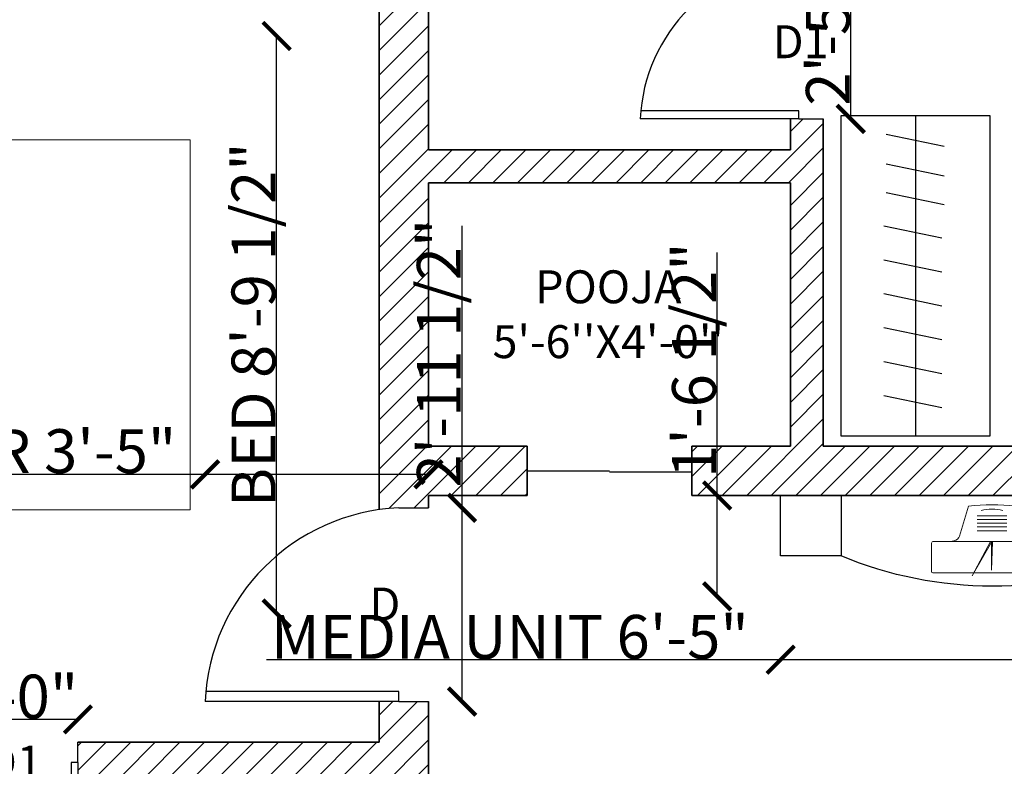
# Model space of a CAD drawing. Units: inches. Extents: x 2094 to 2639, y 1426 to 1997.
# Tile 6 of 8: x 2243 to 2423, y 1730 to 1866. Entities that reach past the tile are written whole.
import ezdxf

# ---------------------------------------------------------------- set-up
doc = ezdxf.new("R2010")
doc.units = ezdxf.units.IN
for name, color, linetype, lineweight in [('A-ANNO-DIMS', 2, 'Continuous', 18), ('A-ANNO-TEXT', 7, 'Continuous', 18), ('A-AREA-IDEN', 7, 'Continuous', 25), ('A-FLOR-CASE', 8, 'Continuous', 25), ('A-FURN', 8, 'Continuous', 18), ('A-WALL-PATT', 8, 'Continuous', 13), ('Doors', 34, 'Continuous', 25), ('Walls', 7, 'Continuous', 35)]:
    doc.layers.add(name, color=color, linetype=linetype, lineweight=lineweight)
doc.layers.add('THIET-BI', color=21, linetype='Continuous')
doc.styles.get("Standard").update_dxf_attribs({"font": 'arial.ttf'})
doc.dimstyles.get("Standard").update_dxf_attribs({"dimtxt": 8, "dimasz": 5, "dimexe": 0.18, "dimexo": 0.0625, "dimgap": 0.09, "dimtad": 1, "dimdec": 1, "dimzin": 0, "dimdsep": 46, "dimlunit": 4, "dimtxsty": 'Standard', "dimblk": 'ARCHTICK', "dimcen": 0.09, "dimse1": 1, "dimse2": 1, "dimadec": 0, "dimazin": 0, "dimtfac": 1, "dimtdec": 1, "dimtofl": 0, "dimtmove": 0, "dimatfit": 3, "dimfxl": 1, "dimtolj": 1, "dimtzin": 0, "dimarcsym": 0})

# ---------------------------------------------------------------- blocks, each defined once
blk = doc.blocks.new('AP0B05')
for p, q in [((35, 100), (35, 880)), ((75, 100), (75, 878.9)), ((35, 100), (35, -20)), ((815, 100), (815, -20))]:
    blk.add_line(p, q)
blk.add_lwpolyline([(35, 100), (75, 100)])
blk.add_arc((-2.4, 62.6), 818.3, 2.6212, 87.3788)
blk = doc.blocks.new('*X3')
at = {"color": 0}
for p, q in [((20.25, 14.8125), (20.2772, 14.8125)), ((20.1875, 14.75), (20.1875, 14.7669)), ((20.199, 14.7812), (20.2772, 14.7812)), ((20.1562, 14.625), (20.1562, 14.7281)), ((20.1739, 14.75), (20.2772, 14.75)), ((20.25, 14.3194), (20.25, 14.75)), ((20.1236, 14.6875), (20.25, 14.6875)), ((20.125, 14.5), (20.125, 14.6893)), ((20.1487, 14.7188), (20.2772, 14.7188)), ((20.0938, 14.375), (20.0938, 14.6504)), ((20.0984, 14.6562), (20.125, 14.6562)), ((20.0625, 14.2573), (20.0625, 14.6116)), ((20.2188, 14.3091), (20.2188, 14.625)), ((20.25, 14.625), (20.2772, 14.625)), ((20.0312, 14.2469), (20.0312, 14.5727)), ((20.125, 14.5938), (20.2772, 14.5938)), ((19.9979, 14.5312), (20.2772, 14.5312)), ((20.023, 14.5625), (20.2772, 14.5625)), ((19.9727, 14.5), (20.25, 14.5)), ((20, 14.2366), (20, 14.5)), ((20.1875, 14.2987), (20.1875, 14.5)), ((19.9476, 14.4688), (20.125, 14.4688)), ((19.9062, 14.375), (19.9062, 14.4174)), ((19.9225, 14.4375), (20, 14.4375)), ((20.125, 14.4062), (20.2772, 14.4062)), ((20.25, 14.4375), (20.2772, 14.4375)), ((19.875, 14.25), (19.875, 14.3785)), ((19.9688, 14.2262), (19.9688, 14.375)), ((20, 14.375), (20.2772, 14.375)), ((20.1562, 14.2884), (20.1562, 14.375)), ((19.8438, 14.1848), (19.8438, 14.3397)), ((19.875, 14.3438), (20.2772, 14.3438)), ((19.8125, 14.1744), (19.8125, 14.3008)), ((19.8219, 14.3125), (20.2291, 14.3125)), ((19.7716, 14.25), (20, 14.25)), ((19.7812, 14.1641), (19.7812, 14.262)), ((19.7967, 14.2812), (20.125, 14.2812)), ((19.9375, 14.2159), (19.9375, 14.25)), ((19.7465, 14.2188), (19.875, 14.2188)), ((19.75, 14.1537), (19.75, 14.2231)), ((19.7213, 14.1875), (19.75, 14.1875)), ((19.7018, 14.0938), (19.7786, 14.0938)), ((19.7188, 14.0726), (19.7188, 14.1136)), ((19.75, 14.0338), (19.75, 14.1032)), ((19.7812, 13.9949), (19.7812, 14.0929)), ((19.7269, 14.0625), (19.8728, 14.0625)), ((19.8125, 14), (19.8125, 14.0825)), ((19.9062, 13.8396), (19.9062, 14.0514)), ((19.752, 14.0312), (19.875, 14.0312)), ((19.9375, 13.8007), (19.9375, 14.0411)), ((19.9688, 13.875), (19.9688, 14.0307)), ((20, 14), (20, 14.0204)), ((19.875, 13.8784), (19.875, 14)), ((19.875, 13.9688), (20.1557, 13.9688)), ((20, 14), (20.0614, 14)), ((20.0625, 13.6454), (20.0625, 13.9996)), ((20.0938, 13.625), (20.0938, 13.9893)), ((20.125, 13.75), (20.125, 13.9789)), ((20.1562, 13.875), (20.1562, 13.9686)), ((19.8275, 13.9375), (20.25, 13.9375)), ((20.25, 13.5), (20.25, 13.9375)), ((19.8526, 13.9062), (20.125, 13.9062)), ((19.8777, 13.875), (20, 13.875)), ((20.0312, 13.6842), (20.0312, 13.875)), ((20.2188, 13.4511), (20.2188, 13.875)), ((20.25, 13.875), (20.2772, 13.875)), ((20, 13.8125), (20.2772, 13.8125)), ((20.125, 13.8438), (20.2772, 13.8438)), ((19.9532, 13.7812), (20.2772, 13.7812)), ((19.9783, 13.75), (20.25, 13.75)), ((20, 13.723), (20, 13.75)), ((20.1875, 13.49), (20.1875, 13.75)), ((20.0035, 13.7188), (20.125, 13.7188)), ((20.25, 13.6875), (20.2772, 13.6875)), ((20.125, 13.6562), (20.2772, 13.6562)), ((20.0789, 13.625), (20.2772, 13.625)), ((20.1562, 13.5288), (20.1562, 13.625)), ((20.104, 13.5938), (20.2772, 13.5938)), ((20.1292, 13.5625), (20.25, 13.5625)), ((20.25, 13.5), (20.2772, 13.5)), ((20.2046, 13.4688), (20.2772, 13.4688)), ((20.2297, 13.4375), (20.2772, 13.4375)), ((20.2549, 13.4062), (20.2772, 13.4062))]:
    blk.add_line(p, q, dxfattribs=at)
blk = doc.blocks.new('MAT-P13')
for p, q in [((-1.17, 0), (-1.17, -0.4)), ((-1.17, 0), (-0.77, 0)), ((-0.77, 0), (-0.77, -0.4)), ((-0.75, 0), (0.75, 0)), ((-0.75, 0), (-0.75, -1.9)), ((0.75, 0), (0.75, -1.9)), ((0.77, 0), (1.17, 0)), ((0.77, 0), (0.77, -0.4)), ((1.17, 0), (1.17, -0.4)), ((-0.7, -0.05), (-0.7, -0.35)), ((-0.7, -0.05), (-0.05, -0.05)), ((-0.05, -0.35), (-0.05, -0.05)), ((0.05, -0.05), (0.7, -0.05)), ((0.05, -0.35), (0.05, -0.05)), ((0.7, -0.05), (0.7, -0.35)), ((-0.7, -0.35), (-0.05, -0.35)), ((0.05, -0.35), (0.7, -0.35)), ((-1.17, -0.4), (-0.77, -0.4)), ((-0.75, -1.0034), (0, -0.4)), ((0, -0.4), (-0.75, -1.0034)), ((0, -0.4), (-0.2, -1.0034)), ((0, -0.4), (0.2, -1.0034)), ((0, -0.4), (0.75, -1.0034)), ((0.77, -0.4), (1.17, -0.4)), ((-0.75, -1.0034), (-0.2, -1.0034)), ((0.2, -1.0034), (0.75, -1.0034)), ((0.75, -1.9), (-0.75, -1.9))]:
    blk.add_line(p, q)
at = {"xscale": -1, "rotation": 90}
blk.add_blockref('*X3', (14.1285, 19.2738), dxfattribs=at)
blk = doc.blocks.new('TVI01')
for p, q in [((-155.1, -10), (-213, -204.9)), ((155.1, -10), (214.2, -208.9)), ((-97.7, -72.9), (99, -72.9)), ((-97.7, -97.9), (99, -97.9)), ((-97.7, -122.9), (99, -122.9)), ((-97.7, -146.1), (99, -146.1)), ((-97.7, -172.9), (99, -172.9)), ((-400, -254.3), (-400, -441.4)), ((-391.8, -243.8), (391.8, -243.8)), ((-3.8, -247.8), (4.2, -432.2)), ((4.2, -247.8), (10.5, -243.6)), ((4.2, -247.8), (130.6, -471.4)), ((4.2, -247.8), (4.2, -432.2)), ((10.5, -243.6), (130.6, -471.4)), ((400, -254.3), (400, -441.4)), ((-391.8, -451.9), (391.8, -451.9))]:
    blk.add_line(p, q)
for centre, radius, start, end in [((0, -1207.7), 1207.7, 82.62163, 97.37837), ((0, -325), 295, 75.74997, 104.25003), ((-390, -253.7), 10, 100.35421, 183.7314), ((-75.1, -1338.2), 1112.5, 99.19763, 100.35421), ((-260.9, -190.6), 50, 279.19763, 343.45736), ((0.2, -247.8), 4, 0, 184.96916), ((260.9, -190.6), 50, 196.54264, 260.80237), ((75.1, -1338.2), 1112.5, 79.64579, 80.80237), ((390, -253.7), 10, 356.2686, 100.69826), ((-390, -442), 10, 176.2686, 259.64579), ((390, -442), 10, 280.35421, 3.7314)]:
    blk.add_arc(centre, radius, start, end)
blk = doc.blocks.new('A$C4C711776')
at = {"layer": 'THIET-BI'}
for p, q in [((180, 2160), (180, 2520)), ((180, 2520), (540, 2520)), ((540, 2160), (180, 2160)), ((180, 360), (180, 0)), ((180, 360), (540, 360)), ((180, 0), (540, 0))]:
    blk.add_line(p, q, dxfattribs=at)
at = {"layer": 'THIET-BI', "extrusion": (0, 0, -1)}
blk.add_ellipse((2340, 1260), major_axis=(1654.6, 1654.6), ratio=1, start_param=3.5322, end_param=4.321782, dxfattribs=at)
at = {"color": 0, "extrusion": (0, 0, -1), "xscale": 0.9000000000014551, "yscale": 0.9000000000014551, "zscale": -0.9, "rotation": 90}
blk.add_blockref('TVI01', (-485.3, 1261.3), dxfattribs=at)
blk = doc.blocks.new('_ArchTick')
at = {"color": 0, "linetype": 'ByBlock', "const_width": 0.15}
blk.add_lwpolyline([(-0.5, -0.5), (0.5, 0.5)], dxfattribs=at)
blk = doc.blocks.new('*D20')
at = {"layer": 'A-ANNO-DIMS', "color": 0, "lineweight": -2, "transparency": 16777216}
blk.add_line((2395.06, 1847.57), (2395.06, 1876.49), dxfattribs=at)
at = {"layer": 'Defpoints', "color": 0, "transparency": 16777216}
for p in [(2390.06, 1876.49), (2395.06, 1876.49), (2390.06, 1847.57)]:
    blk.add_point(p, dxfattribs=at)
at = {"layer": 'A-ANNO-DIMS', "color": 0, "lineweight": -2, "transparency": 16777216, "xscale": 5, "yscale": 5, "zscale": 5}
for p, rotation in [((2395.06, 1876.49), 90), ((2395.06, 1847.57), 270)]:
    blk.add_blockref('_ArchTick', p, dxfattribs=dict(at, rotation=rotation))
at = {"layer": 'A-ANNO-DIMS', "color": 0, "transparency": 16777216, "insert": (2390.89, 1862.03), "char_height": 8, "attachment_point": 5, "rotation": 90}
blk.add_mtext('\\A1;2\'-5"', dxfattribs=at)
blk = doc.blocks.new('*D24')
at = {"layer": 'A-ANNO-DIMS', "color": 0, "lineweight": -2, "transparency": 16777216}
blk.add_line((2254.12, 1738.06), (2230.09, 1738.06), dxfattribs=at)
at = {"layer": 'Defpoints', "color": 0, "transparency": 16777216}
for p in [(2230.09, 1738.06), (2230.09, 1733.9), (2254.12, 1733.9)]:
    blk.add_point(p, dxfattribs=at)
at = {"layer": 'A-ANNO-DIMS', "color": 0, "lineweight": -2, "transparency": 16777216, "xscale": 5, "yscale": 5, "zscale": 5, "rotation": 180}
blk.add_blockref('_ArchTick', (2230.09, 1738.06), dxfattribs=at)
at = {"layer": 'A-ANNO-DIMS', "color": 0, "lineweight": -2, "transparency": 16777216, "xscale": 5, "yscale": 5, "zscale": 5}
blk.add_blockref('_ArchTick', (2254.12, 1738.06), dxfattribs=at)
at = {"layer": 'A-ANNO-DIMS', "color": 0, "transparency": 16777216, "insert": (2242.11, 1742.23), "char_height": 8, "attachment_point": 5}
blk.add_mtext('\\A1;2\'-0"', dxfattribs=at)
blk = doc.blocks.new('*D25')
at = {"layer": 'A-ANNO-DIMS', "color": 0, "lineweight": -2, "transparency": 16777216}
for p, q in [((2277.31, 1782.75), (2214.62, 1782.75)), ((2318.06, 1782.75), (2277.31, 1782.75))]:
    blk.add_line(p, q, dxfattribs=at)
at = {"layer": 'Defpoints', "color": 0, "transparency": 16777216}
for p in [(2277.31, 1782.75), (2277.31, 1776.64), (2318.06, 1776.64)]:
    blk.add_point(p, dxfattribs=at)
at = {"layer": 'A-ANNO-DIMS', "color": 0, "lineweight": -2, "transparency": 16777216, "xscale": 5, "yscale": 5, "zscale": 5, "rotation": 180}
blk.add_blockref('_ArchTick', (2277.31, 1782.75), dxfattribs=at)
at = {"layer": 'A-ANNO-DIMS', "color": 0, "lineweight": -2, "transparency": 16777216, "xscale": 5, "yscale": 5, "zscale": 5}
blk.add_blockref('_ArchTick', (2318.06, 1782.75), dxfattribs=at)
at = {"layer": 'A-ANNO-DIMS', "color": 0, "transparency": 16777216, "insert": (2243.46, 1786.98), "char_height": 8, "attachment_point": 5}
blk.add_mtext('\\A1;DOOR 3\'-5"', dxfattribs=at)
blk = doc.blocks.new('*D26')
at = {"layer": 'A-ANNO-DIMS', "color": 0, "lineweight": -2, "transparency": 16777216}
for p, q in [((2324.17, 1776.64), (2324.17, 1828.08)), ((2324.17, 1741.32), (2324.17, 1776.64))]:
    blk.add_line(p, q, dxfattribs=at)
at = {"layer": 'Defpoints', "color": 0, "transparency": 16777216}
for p in [(2318.06, 1776.64), (2324.17, 1776.64), (2318.06, 1741.32)]:
    blk.add_point(p, dxfattribs=at)
at = {"layer": 'A-ANNO-DIMS', "color": 0, "lineweight": -2, "transparency": 16777216, "xscale": 5, "yscale": 5, "zscale": 5}
for p, rotation in [((2324.17, 1776.64), 90), ((2324.17, 1741.32), 270)]:
    blk.add_blockref('_ArchTick', p, dxfattribs=dict(at, rotation=rotation))
at = {"layer": 'A-ANNO-DIMS', "color": 0, "transparency": 16777216, "insert": (2319.94, 1804.86), "char_height": 8, "attachment_point": 5, "rotation": 90}
blk.add_mtext('\\A1;2\'-11 1/2"', dxfattribs=at)
blk = doc.blocks.new('*D33')
at = {"layer": 'A-ANNO-DIMS', "color": 0, "lineweight": -2, "transparency": 16777216}
blk.add_line((2290.36, 1757.37), (2290.36, 1862.67), dxfattribs=at)
at = {"layer": 'Defpoints', "color": 0, "transparency": 16777216}
for p in [(2274.56, 1862.67), (2290.36, 1862.67), (2274.56, 1757.37)]:
    blk.add_point(p, dxfattribs=at)
at = {"layer": 'A-ANNO-DIMS', "color": 0, "lineweight": -2, "transparency": 16777216, "xscale": 5, "yscale": 5, "zscale": 5}
for p, rotation in [((2290.36, 1862.67), 90), ((2290.36, 1757.37), 270)]:
    blk.add_blockref('_ArchTick', p, dxfattribs=dict(at, rotation=rotation))
at = {"layer": 'A-ANNO-DIMS', "color": 0, "transparency": 16777216, "insert": (2286.13, 1810.02), "char_height": 8, "attachment_point": 5, "rotation": 90}
blk.add_mtext('\\A1;BED 8\'-9 1/2"', dxfattribs=at)
blk = doc.blocks.new('*D34')
at = {"layer": 'A-ANNO-DIMS', "color": 0, "lineweight": -2, "transparency": 16777216}
blk.add_line((2274.56, 1878.47), (2189.06, 1878.47), dxfattribs=at)
at = {"layer": 'Defpoints', "color": 0, "transparency": 16777216}
for p in [(2189.06, 1878.47), (2189.06, 1862.67), (2274.56, 1862.67)]:
    blk.add_point(p, dxfattribs=at)
at = {"layer": 'A-ANNO-DIMS', "color": 0, "lineweight": -2, "transparency": 16777216, "xscale": 5, "yscale": 5, "zscale": 5, "rotation": 180}
blk.add_blockref('_ArchTick', (2189.06, 1878.47), dxfattribs=at)
at = {"layer": 'A-ANNO-DIMS', "color": 0, "lineweight": -2, "transparency": 16777216, "xscale": 5, "yscale": 5, "zscale": 5}
blk.add_blockref('_ArchTick', (2274.56, 1878.47), dxfattribs=at)
at = {"layer": 'A-ANNO-DIMS', "color": 0, "transparency": 16777216, "insert": (2231.81, 1882.7), "char_height": 8, "attachment_point": 5}
blk.add_mtext('\\A1;7\'-1 1/2"', dxfattribs=at)
blk = doc.blocks.new('*D49')
at = {"layer": 'A-ANNO-DIMS', "color": 0, "lineweight": -2, "transparency": 16777216}
for p, q in [((2382.28, 1748.95), (2288.52, 1748.95)), ((2459.46, 1748.95), (2382.28, 1748.95))]:
    blk.add_line(p, q, dxfattribs=at)
at = {"layer": 'Defpoints', "color": 0, "transparency": 16777216}
for p in [(2382.28, 1760.52), (2459.46, 1760.52), (2382.28, 1748.95)]:
    blk.add_point(p, dxfattribs=at)
at = {"layer": 'A-ANNO-DIMS', "color": 0, "lineweight": -2, "transparency": 16777216, "xscale": 5, "yscale": 5, "zscale": 5, "rotation": 180}
blk.add_blockref('_ArchTick', (2382.28, 1748.95), dxfattribs=at)
at = {"layer": 'A-ANNO-DIMS', "color": 0, "lineweight": -2, "transparency": 16777216, "xscale": 5, "yscale": 5, "zscale": 5}
blk.add_blockref('_ArchTick', (2459.46, 1748.95), dxfattribs=at)
at = {"layer": 'A-ANNO-DIMS', "color": 0, "transparency": 16777216, "insert": (2332.9, 1753.12), "char_height": 8, "attachment_point": 5}
blk.add_mtext('\\A1;MEDIA UNIT 6\'-5"', dxfattribs=at)
blk = doc.blocks.new('*D50')
at = {"layer": 'A-ANNO-DIMS', "color": 0, "lineweight": -2, "transparency": 16777216}
for p, q in [((2370.7, 1778.9), (2370.7, 1823.23)), ((2370.7, 1760.52), (2370.7, 1778.9))]:
    blk.add_line(p, q, dxfattribs=at)
at = {"layer": 'Defpoints', "color": 0, "transparency": 16777216}
for p in [(2370.7, 1778.9), (2382.28, 1778.9), (2382.28, 1760.52)]:
    blk.add_point(p, dxfattribs=at)
at = {"layer": 'A-ANNO-DIMS', "color": 0, "lineweight": -2, "transparency": 16777216, "xscale": 5, "yscale": 5, "zscale": 5}
for p, rotation in [((2370.7, 1778.9), 90), ((2370.7, 1760.52), 270)]:
    blk.add_blockref('_ArchTick', p, dxfattribs=dict(at, rotation=rotation))
at = {"layer": 'A-ANNO-DIMS', "color": 0, "transparency": 16777216, "insert": (2366.47, 1803.57), "char_height": 8, "attachment_point": 5, "rotation": 90}
blk.add_mtext('\\A1;1\'-6 1/2"', dxfattribs=at)
blk = doc.blocks.new('*D66')
at = {"layer": 'A-ANNO-DIMS', "color": 0, "lineweight": -2, "transparency": 16777216}
blk.add_line((2336.06, 1954.65), (2366.06, 1954.65), dxfattribs=at)
at = {"layer": 'Defpoints', "color": 0, "transparency": 16777216}
for p in [(2366.06, 1954.65), (2336.06, 1787.9), (2366.06, 1787.9)]:
    blk.add_point(p, dxfattribs=at)
at = {"layer": 'A-ANNO-DIMS', "color": 0, "lineweight": -2, "transparency": 16777216, "xscale": 5, "yscale": 5, "zscale": 5, "rotation": 180}
blk.add_blockref('_ArchTick', (2336.06, 1954.65), dxfattribs=at)
at = {"layer": 'A-ANNO-DIMS', "color": 0, "lineweight": -2, "transparency": 16777216, "xscale": 5, "yscale": 5, "zscale": 5}
blk.add_blockref('_ArchTick', (2366.06, 1954.65), dxfattribs=at)
at = {"layer": 'A-ANNO-DIMS', "color": 0, "transparency": 16777216, "insert": (2351.06, 1958.82), "char_height": 8, "attachment_point": 5}
blk.add_mtext('\\A1;2\'-6"', dxfattribs=at)
blk = doc.blocks.new('*D76')
at = {"layer": 'A-ANNO-DIMS', "color": 0, "lineweight": -2, "transparency": 16777216}
blk.add_line((2248.06, 1954.65), (2318.06, 1954.65), dxfattribs=at)
at = {"layer": 'Defpoints', "color": 0, "transparency": 16777216}
for p in [(2318.06, 1954.65), (2248.06, 1468.9), (2318.06, 1468.9)]:
    blk.add_point(p, dxfattribs=at)
at = {"layer": 'A-ANNO-DIMS', "color": 0, "lineweight": -2, "transparency": 16777216, "xscale": 5, "yscale": 5, "zscale": 5, "rotation": 180}
blk.add_blockref('_ArchTick', (2248.06, 1954.65), dxfattribs=at)
at = {"layer": 'A-ANNO-DIMS', "color": 0, "lineweight": -2, "transparency": 16777216, "xscale": 5, "yscale": 5, "zscale": 5}
blk.add_blockref('_ArchTick', (2318.06, 1954.65), dxfattribs=at)
at = {"layer": 'A-ANNO-DIMS', "color": 0, "transparency": 16777216, "insert": (2283.06, 1958.82), "char_height": 8, "attachment_point": 5}
blk.add_mtext('\\A1;5\'-10"', dxfattribs=at)
blk = doc.blocks.new('*D77')
at = {"layer": 'A-ANNO-DIMS', "color": 0, "lineweight": -2, "transparency": 16777216}
for p, q in [((2308.06, 1954.65), (2318.06, 1954.65)), ((2318.06, 1954.65), (2350.72, 1954.65))]:
    blk.add_line(p, q, dxfattribs=at)
at = {"layer": 'Defpoints', "color": 0, "transparency": 16777216}
for p in [(2318.06, 1954.65), (2308.06, 1468.9), (2318.06, 1468.9)]:
    blk.add_point(p, dxfattribs=at)
at = {"layer": 'A-ANNO-DIMS', "color": 0, "lineweight": -2, "transparency": 16777216, "xscale": 5, "yscale": 5, "zscale": 5, "rotation": 180}
blk.add_blockref('_ArchTick', (2308.06, 1954.65), dxfattribs=at)
at = {"layer": 'A-ANNO-DIMS', "color": 0, "lineweight": -2, "transparency": 16777216, "xscale": 5, "yscale": 5, "zscale": 5}
blk.add_blockref('_ArchTick', (2318.06, 1954.65), dxfattribs=at)
at = {"layer": 'A-ANNO-DIMS', "color": 0, "transparency": 16777216, "insert": (2336.89, 1958.82), "char_height": 8, "attachment_point": 5}
blk.add_mtext('\\A1;0\'-10"', dxfattribs=at)
blk = doc.blocks.new('*D79')
at = {"layer": 'A-ANNO-DIMS', "color": 0, "lineweight": -2, "transparency": 16777216}
for p, q in [((2562.81, 1741.32), (2562.81, 1786.41)), ((2562.81, 1733.9), (2562.81, 1741.32))]:
    blk.add_line(p, q, dxfattribs=at)
at = {"layer": 'Defpoints', "color": 0, "transparency": 16777216}
for p in [(2309.06, 1741.32), (2562.81, 1741.32), (2309.06, 1733.9)]:
    blk.add_point(p, dxfattribs=at)
at = {"layer": 'A-ANNO-DIMS', "color": 0, "lineweight": -2, "transparency": 16777216, "xscale": 5, "yscale": 5, "zscale": 5}
for p, rotation in [((2562.81, 1741.32), 90), ((2562.81, 1733.9), 270)]:
    blk.add_blockref('_ArchTick', p, dxfattribs=dict(at, rotation=rotation))
at = {"layer": 'A-ANNO-DIMS', "color": 0, "transparency": 16777216, "insert": (2558.58, 1766.37), "char_height": 8, "attachment_point": 5, "rotation": 90}
blk.add_mtext('\\A1;0\'-7 1/2"', dxfattribs=at)
blk = doc.blocks.new('*D80')
at = {"layer": 'A-ANNO-DIMS', "color": 0, "lineweight": -2, "transparency": 16777216}
for p, q in [((2318.06, 1954.65), (2336.06, 1954.65)), ((2336.06, 1954.65), (2361.75, 1954.65))]:
    blk.add_line(p, q, dxfattribs=at)
at = {"layer": 'Defpoints', "color": 0, "transparency": 16777216}
for p in [(2336.06, 1954.65), (2318.06, 1787.9), (2336.06, 1787.9)]:
    blk.add_point(p, dxfattribs=at)
at = {"layer": 'A-ANNO-DIMS', "color": 0, "lineweight": -2, "transparency": 16777216, "xscale": 5, "yscale": 5, "zscale": 5, "rotation": 180}
blk.add_blockref('_ArchTick', (2318.06, 1954.65), dxfattribs=at)
at = {"layer": 'A-ANNO-DIMS', "color": 0, "lineweight": -2, "transparency": 16777216, "xscale": 5, "yscale": 5, "zscale": 5}
blk.add_blockref('_ArchTick', (2336.06, 1954.65), dxfattribs=at)
at = {"layer": 'A-ANNO-DIMS', "color": 0, "transparency": 16777216, "insert": (2351.4, 1958.82), "char_height": 8, "attachment_point": 5}
blk.add_mtext('\\A1;1\'-6"', dxfattribs=at)
blk = doc.blocks.new('*D81')
at = {"layer": 'A-ANNO-DIMS', "color": 0, "lineweight": -2, "transparency": 16777216}
for p, q in [((2249.13, 1954.65), (2257.66, 1954.65)), ((2257.66, 1954.65), (2302.74, 1954.65))]:
    blk.add_line(p, q, dxfattribs=at)
at = {"layer": 'Defpoints', "color": 0, "transparency": 16777216}
for p in [(2257.66, 1954.65), (2249.13, 1589.48), (2257.66, 1589.48)]:
    blk.add_point(p, dxfattribs=at)
at = {"layer": 'A-ANNO-DIMS', "color": 0, "lineweight": -2, "transparency": 16777216, "xscale": 5, "yscale": 5, "zscale": 5, "rotation": 180}
blk.add_blockref('_ArchTick', (2249.13, 1954.65), dxfattribs=at)
at = {"layer": 'A-ANNO-DIMS', "color": 0, "lineweight": -2, "transparency": 16777216, "xscale": 5, "yscale": 5, "zscale": 5}
blk.add_blockref('_ArchTick', (2257.66, 1954.65), dxfattribs=at)
at = {"layer": 'A-ANNO-DIMS', "color": 0, "transparency": 16777216, "insert": (2282.7, 1958.87), "char_height": 8, "attachment_point": 5}
blk.add_mtext('\\A1;0\'-8 1/2"', dxfattribs=at)
blk = doc.blocks.new('*D83')
at = {"layer": 'A-ANNO-DIMS', "color": 0, "lineweight": -2, "transparency": 16777216}
for p, q in [((2249.25, 1954.65), (2257.43, 1954.65)), ((2257.43, 1954.65), (2283.88, 1954.65))]:
    blk.add_line(p, q, dxfattribs=at)
at = {"layer": 'Defpoints', "color": 0, "transparency": 16777216}
for p in [(2257.43, 1954.65), (2249.25, 1595.79), (2257.43, 1595.79)]:
    blk.add_point(p, dxfattribs=at)
at = {"layer": 'A-ANNO-DIMS', "color": 0, "lineweight": -2, "transparency": 16777216, "xscale": 5, "yscale": 5, "zscale": 5, "rotation": 180}
blk.add_blockref('_ArchTick', (2249.25, 1954.65), dxfattribs=at)
at = {"layer": 'A-ANNO-DIMS', "color": 0, "lineweight": -2, "transparency": 16777216, "xscale": 5, "yscale": 5, "zscale": 5}
blk.add_blockref('_ArchTick', (2257.43, 1954.65), dxfattribs=at)
at = {"layer": 'A-ANNO-DIMS', "color": 0, "transparency": 16777216, "insert": (2273.16, 1958.82), "char_height": 8, "attachment_point": 5}
blk.add_mtext('\\A1;0\'-8"', dxfattribs=at)

msp = doc.modelspace()

# ---------------------------------------------------------------- hatches: boundary and pattern name
at = {"layer": 'A-WALL-PATT', "transparency": 33554585}
h = msp.add_hatch(dxfattribs=at)
h.set_pattern_fill('ANSI31', color=256)
h.paths.add_polyline_path([(2189.06, 1727.9), (2230.3, 1727.9, -0.022928), (2230.09, 1730.2), (2230.09, 1733.9), (2189.06, 1733.9), (2189.06, 1742.37), (2180.06, 1742.37), (2180.06, 1714.4), (2189.06, 1714.4)])
h.paths.add_polyline_path([(2456.51, 1574.9), (2413.83, 1574.9), (2413.83, 1565.9), (2456.51, 1565.9)])
h.paths.add_polyline_path([(2537.06, 1643.81), (2528.06, 1643.81), (2528.06, 1574.9), (2519.78, 1574.9), (2519.78, 1571.88), (2519.78, 1565.9), (2537.06, 1565.9)])
h.paths.add_polyline_path([(2339.06, 1928.9), (2300.94, 1928.9), (2300.94, 1919.9), (2309.06, 1919.9), (2309.06, 1776.3, -0.024186), (2312.62, 1776.64), (2318.06, 1776.64), (2318.06, 1778.9), (2336.06, 1778.9), (2336.06, 1787.9), (2318.06, 1787.9), (2318.06, 1835.9), (2384.06, 1835.9), (2384.06, 1787.9), (2366.06, 1787.9), (2366.06, 1778.9), (2479.64, 1778.9), (2479.64, 1784.88, -0.018603), (2479.89, 1787.9), (2390.06, 1787.9), (2390.06, 1847.57), (2385.61, 1847.57), (2384.06, 1847.57), (2384.06, 1841.9), (2318.06, 1841.9), (2318.06, 1919.9), (2339.06, 1919.9)])
h.paths.add_polyline_path([(2252.94, 1928.9), (2180.06, 1928.9), (2180.06, 1790.37), (2189.06, 1790.37), (2189.06, 1843.77), (2189.06, 1919.9), (2252.94, 1919.9)])
h.paths.add_polyline_path([(2472.33, 1928.9), (2363.06, 1928.9), (2363.06, 1919.9), (2384.06, 1919.9), (2384.06, 1876.38, -0.012802), (2385.61, 1876.49), (2390.06, 1876.49), (2390.06, 1919.9), (2472.33, 1919.9)], flags=17)
h.paths.add_polyline_path([(2537.06, 1928.9), (2520.33, 1928.9), (2520.33, 1919.9), (2528.06, 1919.9), (2528.06, 1905.95), (2528.06, 1787.9), (2518.5, 1787.9), (2518.5, 1784.88), (2518.5, 1778.9), (2528.06, 1778.9), (2528.06, 1715.81), (2537.06, 1715.81)])
h.paths.add_polyline_path([(2379.33, 1857.12), (2393.06, 1857.12), (2393.06, 1866.16), (2379.33, 1866.16)], flags=25)
h.paths.add_polyline_path([(2235.85, 1725.77), (2249.57, 1725.77), (2249.57, 1734.81), (2235.85, 1734.81)], flags=25)
h.paths.add_polyline_path([(2305.79, 1754.6), (2314.84, 1754.6), (2314.84, 1763.6), (2305.79, 1763.6)], flags=9)
h.paths.add_polyline_path([(2493.85, 1778.22), (2502.9, 1778.22), (2502.9, 1787.22), (2493.85, 1787.22)], flags=9)
h.paths.add_polyline_path([(2370.69, 1555.65), (2381.6, 1555.65), (2381.6, 1564.65), (2370.69, 1564.65)], flags=9)
h.paths.add_polyline_path([(2461.57, 1555.65), (2477.6, 1555.65), (2477.6, 1564.65), (2461.57, 1564.65)], flags=9)
h.paths.add_polyline_path([(2493.18, 1565.15), (2509.22, 1565.15), (2509.22, 1574.15), (2493.18, 1574.15)], flags=9)
h.paths.add_polyline_path([(2408.32, 1501.7), (2449.12, 1501.7), (2449.12, 1520.36), (2408.32, 1520.36)], flags=9)
h.paths.add_polyline_path([(2398.49, 1698.6), (2441.61, 1698.6), (2441.61, 1717.26), (2398.49, 1717.26)], flags=9)
h.paths.add_polyline_path([(2248.63, 1683.29), (2287.87, 1683.29), (2287.87, 1701.95), (2248.63, 1701.95)], flags=25)
h.paths.add_polyline_path([(2440.73, 1823.2), (2483.86, 1823.2), (2483.86, 1841.85), (2440.73, 1841.85)], flags=9)
h.paths.add_polyline_path([(2335.3, 1804.5), (2370.65, 1804.5), (2370.65, 1823.15), (2335.3, 1823.15)], flags=25)
h.paths.add_polyline_path([(2335.3, 1893.12), (2370.65, 1893.12), (2370.65, 1911.77), (2335.3, 1911.77)], flags=25)
h.paths.add_polyline_path([(2241.82, 1863.6), (2290.11, 1863.6), (2290.11, 1882.25), (2241.82, 1882.25)], flags=9)
h = msp.add_hatch(dxfattribs=at)
h.set_pattern_fill('ANSI31', color=256)
h.paths.add_polyline_path([(2318.06, 1741.32), (2312.62, 1741.32), (2309.06, 1741.32), (2309.06, 1733.9), (2254.12, 1733.9), (2254.12, 1730.2), (2254.12, 1727.9), (2309.06, 1727.9), (2309.06, 1676.9), (2189.06, 1676.9), (2189.06, 1690.4), (2180.06, 1690.4), (2180.06, 1646.9), (2189.06, 1646.9), (2189.06, 1670.9), (2309.06, 1670.9), (2309.06, 1640.9), (2318.06, 1640.9)])
h.paths.add_polyline_path([(2318.06, 1604.9), (2309.06, 1604.9), (2309.06, 1574.9), (2189.06, 1574.9), (2189.06, 1598.9), (2180.06, 1598.9), (2180.06, 1459.9), (2318.06, 1459.9), (2318.06, 1468.9), (2189.06, 1468.9), (2189.06, 1565.9), (2341.83, 1565.9), (2341.83, 1574.9), (2318.06, 1574.9)])

# ---------------------------------------------------------------- linework, layer by layer
at = {"layer": 'A-FLOR-CASE'}
for p, q in [((2406.88, 1848.21), (2406.88, 1789.69)), ((2412.1, 1842.53), (2401.55, 1844.73)), ((2412.1, 1837.1), (2401.55, 1839.3)), ((2412.1, 1831.88), (2401.55, 1834.08)), ((2411.68, 1825.81), (2401.12, 1828.02)), ((2411.68, 1819.63), (2401.12, 1821.83)), ((2411.68, 1813.44), (2401.12, 1815.64)), ((2411.68, 1807.25), (2401.12, 1809.45)), ((2411.68, 1801.07), (2401.12, 1803.27)), ((2411.68, 1794.88), (2401.12, 1797.08))]:
    msp.add_line(p, q, dxfattribs=at)
msp.add_lwpolyline([(2420.45, 1848.21), (2420.45, 1789.69), (2393.31, 1789.69), (2393.31, 1848.21)], close=True, dxfattribs=at)
at = {"layer": 'Doors'}
for p, q in [((2336.06, 1783.4), (2351.06, 1783.4)), ((2351.06, 1783.23), (2366.06, 1783.23))]:
    msp.add_line(p, q, dxfattribs=at)
at = {"layer": 'Walls'}
for p, q in [((2309.06, 1919.9), (2309.06, 1776.3)), ((2318.06, 1919.9), (2318.06, 1841.9)), ((2384.06, 1847.57), (2384.06, 1841.9)), ((2390.06, 1847.57), (2390.06, 1787.9)), ((2318.06, 1841.9), (2384.06, 1841.9)), ((2318.06, 1835.9), (2384.06, 1835.9)), ((2318.06, 1835.9), (2318.06, 1787.9)), ((2384.06, 1835.9), (2384.06, 1787.9)), ((2318.06, 1787.9), (2336.06, 1787.9)), ((2336.06, 1787.9), (2336.06, 1778.9)), ((2366.06, 1787.9), (2366.06, 1778.9)), ((2366.06, 1787.9), (2384.06, 1787.9)), ((2390.06, 1787.9), (2479.89, 1787.9)), ((2318.06, 1778.9), (2336.06, 1778.9)), ((2318.06, 1778.9), (2318.06, 1776.64)), ((2366.06, 1778.9), (2479.64, 1778.9)), ((2309.06, 1741.32), (2309.06, 1733.9)), ((2318.06, 1741.32), (2318.06, 1640.9)), ((2254.12, 1733.9), (2309.06, 1733.9))]:
    msp.add_line(p, q, dxfattribs=at)

# ---------------------------------------------------------------- block references
at = {"layer": 'A-FURN'}
for name, p, xscale, yscale, zscale, rotation in [('MAT-P13', (2189.06, 1810.02), 45.00172282535224, 45.00172282535224, 45.00172282535224, 90), ('A$C4C711776', (2459.46, 1762.36), 0.0306262109582552, 0.0306262109582552, 0.0306262109582552, 89.99999999999991)]:
    msp.add_blockref(name, p, dxfattribs=dict(at, xscale=xscale, yscale=yscale, zscale=zscale, rotation=rotation))
at = {"layer": 'Doors'}
for p, xscale, yscale, zscale, rotation in [((2389.31, 1846.27), 0.0370855999522285, 0.0370855999522285, 0.0370855999522285, 90), ((2317.15, 1739.74), 0.0452790538864669, 0.0452790538864669, 0.0452790538864669, 89.99999999999999), ((2255.2, 1733.28), 0.0308176600246466, 0.0308176600246466, 0.0308176600246466, 180)]:
    msp.add_blockref('AP0B05', p, dxfattribs=dict(at, xscale=xscale, yscale=yscale, zscale=zscale, rotation=rotation))

# ---------------------------------------------------------------- texts
at = {"layer": 'A-ANNO-TEXT'}
for s, p in [('D1', (2380.84, 1858.63)), ('D', (2307.29, 1756.1)), ('D1', (2237.35, 1727.28))]:
    msp.add_text(s, height=6, dxfattribs=at).set_placement(p)
at = {"layer": 'A-AREA-IDEN', "insert": (2324.29, 1819.95), "char_height": 6, "attachment_point": 1}
msp.add_mtext_dynamic_manual_height_columns("\\pxqc;POOJA\\P5'-6''X4'-0''", width=53.0999, gutter_width=63.55, heights=[0], dxfattribs=at)

# ---------------------------------------------------------------- dimensions: what is measured, and where the dimension line sits
at = {"layer": 'A-ANNO-DIMS'}
for base, p1, p2, picture, middle in [((2257.66, 1954.65), (2249.13, 1589.48), (2257.66, 1589.48), '*D81', (2282.7, 1958.87)), ((2318.06, 1954.65), (2248.06, 1468.9), (2318.06, 1468.9), '*D76', (2283.06, 1958.82)), ((2257.43, 1954.65), (2249.25, 1595.79), (2257.43, 1595.79), '*D83', (2273.16, 1958.82)), ((2318.06, 1954.65), (2308.06, 1468.9), (2318.06, 1468.9), '*D77', (2336.89, 1958.82)), ((2336.06, 1954.65), (2318.06, 1787.9), (2336.06, 1787.9), '*D80', (2351.4, 1958.82)), ((2366.06, 1954.65), (2336.06, 1787.9), (2366.06, 1787.9), '*D66', (2351.06, 1958.82))]:
    dim = msp.add_linear_dim(base=base, p1=p1, p2=p2, dimstyle='Standard', override={"dimdec": 1, "dimlfac": 1, "dimrnd": 0, "dimzin": 1, "dimdsep": 46, "dimlunit": 4, "dimfrac": 2}, dxfattribs=at)
    dim.commit()
    dim.dimension.update_dxf_attribs({"geometry": picture, "text_midpoint": middle})
for base, p1, p2, angle, picture, middle in [((2189.06, 1878.47), (2274.56, 1862.67), (2189.06, 1862.67), 180, '*D34', (2231.81, 1882.7)), ((2395.06, 1876.49), (2390.06, 1847.57), (2390.06, 1876.49), 90, '*D20', (2390.89, 1862.03)), ((2324.17, 1776.64), (2318.06, 1741.32), (2318.06, 1776.64), 90, '*D26', (2319.94, 1804.86)), ((2370.7, 1778.9), (2382.28, 1760.52), (2382.28, 1778.9), 90, '*D50', (2366.47, 1803.57)), ((2562.81, 1741.32), (2309.06, 1733.9), (2309.06, 1741.32), 90, '*D79', (2558.58, 1766.37)), ((2230.09, 1738.06), (2254.12, 1733.9), (2230.09, 1733.9), 180, '*D24', (2242.11, 1742.23))]:
    dim = msp.add_linear_dim(base=base, p1=p1, p2=p2, angle=angle, dimstyle='Standard', override={"dimdec": 1, "dimlfac": 1, "dimrnd": 0, "dimzin": 1, "dimdsep": 46, "dimlunit": 4, "dimfrac": 2}, dxfattribs=at)
    dim.commit()
    dim.dimension.update_dxf_attribs({"geometry": picture, "text_midpoint": middle})
for base, p1, p2, angle, text, picture, middle in [((2290.36, 1862.67), (2274.56, 1757.37), (2274.56, 1862.67), 90, 'BED <>', '*D33', (2286.13, 1810.02)), ((2277.3052, 1782.7522), (2318.0563, 1776.6396), (2277.3052, 1776.6396), 180, 'DOOR <>', '*D25', (2243.4648, 1786.9841)), ((2382.28, 1748.95), (2459.46, 1760.52), (2382.28, 1760.52), 180, 'MEDIA UNIT <>', '*D49', (2332.9, 1753.12))]:
    dim = msp.add_linear_dim(base=base, p1=p1, p2=p2, angle=angle, text=text, dimstyle='Standard', override={"dimdec": 1, "dimlfac": 1, "dimrnd": 0, "dimzin": 1, "dimdsep": 46, "dimlunit": 4, "dimfrac": 2}, dxfattribs=at)
    dim.commit()
    dim.dimension.update_dxf_attribs({"geometry": picture, "text_midpoint": middle})

doc.saveas('drawing.dxf')
